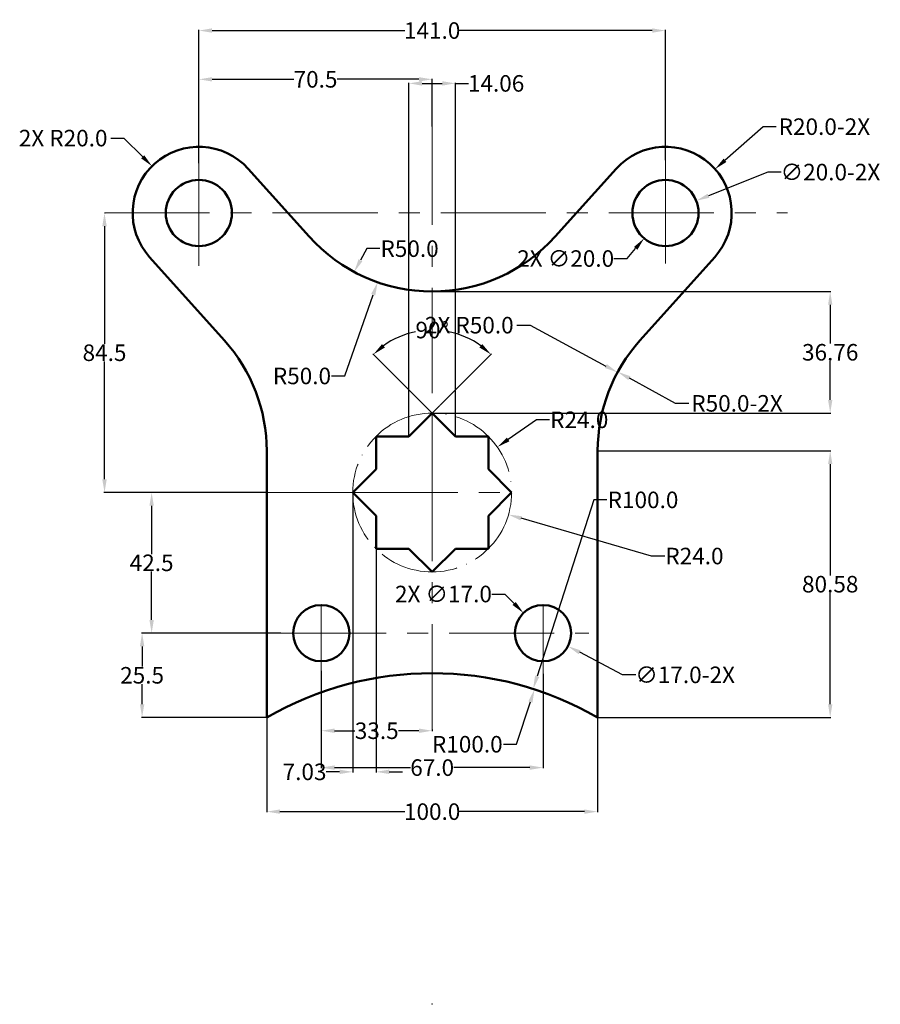
# Model space of a CAD drawing. Units: inches. Extents: x 181 to 441, y 19 to 317.
import ezdxf

# ---------------------------------------------------------------- set-up
doc = ezdxf.new("R2010")
doc.units = ezdxf.units.IN
doc.header["$MEASUREMENT"] = 0
doc.linetypes.add('ACAD_ISO04W100', pattern=[30, 24, -3, 0, -3])
doc.linetypes.add('CENTER', pattern=[50.8, 31.75, -6.35, 6.35, -6.35])
for name, color, linetype, lineweight in [('M-CNTR', 4, 'CENTER', 18), ('M-CONS', 4, 'ACAD_ISO04W100', 13), ('M-DIMS', 2, 'Continuous', 25), ('M-OUTL', 7, 'Continuous', 50)]:
    doc.layers.add(name, color=color, linetype=linetype, lineweight=lineweight)
doc.styles.get("Standard").update_dxf_attribs({"font": 'arial.ttf'})
doc.dimstyles.get("Standard").update_dxf_attribs({"dimtxt": 5, "dimasz": 4, "dimexe": 0.18, "dimexo": 0.0625, "dimgap": 0.09, "dimtad": 0, "dimtih": 1, "dimtoh": 1, "dimdec": 1, "dimzin": 0, "dimdsep": 46, "dimtxsty": 'Standard', "dimcen": 0.09, "dimadec": 0, "dimazin": 0, "dimtfac": 1, "dimtdec": 1, "dimtofl": 0, "dimtmove": 0, "dimatfit": 3, "dimfxl": 1, "dimtolj": 1, "dimtzin": 0, "dimarcsym": 0})

# ---------------------------------------------------------------- blocks, each defined once
blk = doc.blocks.new('*D1')
at = {"layer": 'Defpoints', "color": 0, "transparency": 16777216}
for p in [(336.36, 114.2), (305.44, 19.1)]:
    blk.add_point(p, dxfattribs=at)
at = {"layer": 'M-DIMS', "color": 0, "lineweight": -2, "transparency": 16777216}
for p, q in [((330.97, 97.61), (335.12, 110.39)), ((326.97, 97.61), (330.97, 97.61))]:
    blk.add_line(p, q, dxfattribs=at)
at = {"layer": 'M-DIMS', "color": 0, "transparency": 16777216}
blk.add_solid([(334.49, 110.6), (335.75, 110.19), (336.36, 114.2)], dxfattribs=at)
at = {"layer": 'M-DIMS', "color": 0, "transparency": 16777216, "insert": (316.06, 97.61), "char_height": 5, "attachment_point": 5}
blk.add_mtext('\\A1;R100.0', dxfattribs=at)
blk = doc.blocks.new('*D2')
at = {"layer": 'Defpoints', "color": 0, "transparency": 16777216}
for p in [(271.94, 119.92), (271.94, 101.7), (305.44, 102.17)]:
    blk.add_point(p, dxfattribs=at)
at = {"layer": 'M-DIMS', "color": 0, "lineweight": -2, "transparency": 16777216}
for p, q in [((271.94, 119.85), (271.94, 101.52)), ((275.94, 101.7), (282.09, 101.7)), ((301.44, 101.7), (295.29, 101.7)), ((305.44, 102.11), (305.44, 101.52))]:
    blk.add_line(p, q, dxfattribs=at)
at = {"layer": 'M-DIMS', "color": 0, "transparency": 16777216}
for points in [[(275.94, 102.36), (275.94, 101.03), (271.94, 101.7)], [(301.44, 102.36), (301.44, 101.03), (305.44, 101.7)]]:
    blk.add_solid(points, dxfattribs=at)
at = {"layer": 'M-DIMS', "color": 0, "transparency": 16777216, "insert": (288.69, 101.7), "char_height": 5, "attachment_point": 5}
blk.add_mtext('\\A1;33.5', dxfattribs=at)
blk = doc.blocks.new('*D3')
at = {"layer": 'Defpoints', "color": 0, "transparency": 16777216}
for p in [(271.94, 119.92), (338.94, 118.97), (338.94, 90.55)]:
    blk.add_point(p, dxfattribs=at)
at = {"layer": 'M-DIMS', "color": 0, "lineweight": -2, "transparency": 16777216}
for p, q in [((271.94, 119.85), (271.94, 90.37)), ((338.94, 118.91), (338.94, 90.37)), ((275.94, 90.55), (298.85, 90.55)), ((334.94, 90.55), (312.03, 90.55))]:
    blk.add_line(p, q, dxfattribs=at)
at = {"layer": 'M-DIMS', "color": 0, "transparency": 16777216}
for points in [[(275.94, 91.22), (275.94, 89.89), (271.94, 90.55)], [(334.94, 91.22), (334.94, 89.89), (338.94, 90.55)]]:
    blk.add_solid(points, dxfattribs=at)
at = {"layer": 'M-DIMS', "color": 0, "transparency": 16777216, "insert": (305.44, 90.55), "char_height": 5, "attachment_point": 5}
blk.add_mtext('\\A1;67.0', dxfattribs=at)
blk = doc.blocks.new('*D4')
at = {"layer": 'Defpoints', "color": 0, "transparency": 16777216}
for p in [(255.44, 105.7), (355.44, 105.7), (355.44, 77.24)]:
    blk.add_point(p, dxfattribs=at)
at = {"layer": 'M-DIMS', "color": 0, "lineweight": -2, "transparency": 16777216}
for p, q in [((255.44, 105.64), (255.44, 77.06)), ((355.44, 105.64), (355.44, 77.06)), ((259.44, 77.24), (297.16, 77.24)), ((351.44, 77.24), (313.73, 77.24))]:
    blk.add_line(p, q, dxfattribs=at)
at = {"layer": 'M-DIMS', "color": 0, "transparency": 16777216}
for points in [[(259.44, 77.91), (259.44, 76.58), (255.44, 77.24)], [(351.44, 77.91), (351.44, 76.58), (355.44, 77.24)]]:
    blk.add_solid(points, dxfattribs=at)
at = {"layer": 'M-DIMS', "color": 0, "transparency": 16777216, "insert": (305.44, 77.24), "char_height": 5, "attachment_point": 5}
blk.add_mtext('\\A1;100.0', dxfattribs=at)
blk = doc.blocks.new('*D5')
at = {"layer": 'Defpoints', "color": 0, "transparency": 16777216}
for p in [(331.41, 135.14), (346.47, 127.25)]:
    blk.add_point(p, dxfattribs=at)
at = {"layer": 'M-DIMS', "color": 0, "lineweight": -2, "transparency": 16777216}
for p, q in [((338.85, 131.2), (339.03, 131.2)), ((338.94, 131.11), (338.94, 131.29)), ((363, 118.59), (350.02, 125.4)), ((367, 118.59), (363, 118.59))]:
    blk.add_line(p, q, dxfattribs=at)
at = {"layer": 'M-DIMS', "color": 0, "transparency": 16777216}
blk.add_solid([(350.32, 125.99), (349.71, 124.81), (346.47, 127.25)], dxfattribs=at)
at = {"layer": 'M-DIMS', "color": 0, "transparency": 16777216, "insert": (381.88, 118.59), "char_height": 5, "attachment_point": 5}
blk.add_mtext('\\A1;∅17.0-2X', dxfattribs=at)
blk = doc.blocks.new('*D6')
at = {"layer": 'Defpoints', "color": 0, "transparency": 16777216}
for p in [(217.79, 131.2), (259.75, 131.2), (255.44, 105.7)]:
    blk.add_point(p, dxfattribs=at)
at = {"layer": 'M-DIMS', "color": 0, "lineweight": -2, "transparency": 16777216}
for p, q in [((259.69, 131.2), (217.61, 131.2)), ((217.79, 127.2), (217.79, 121.09)), ((217.79, 109.7), (217.79, 115.81)), ((255.38, 105.7), (217.61, 105.7))]:
    blk.add_line(p, q, dxfattribs=at)
at = {"layer": 'M-DIMS', "color": 0, "transparency": 16777216}
for points in [[(217.13, 127.2), (218.46, 127.2), (217.79, 131.2)], [(217.13, 109.7), (218.46, 109.7), (217.79, 105.7)]]:
    blk.add_solid(points, dxfattribs=at)
at = {"layer": 'M-DIMS', "color": 0, "transparency": 16777216, "insert": (217.79, 118.45), "char_height": 5, "attachment_point": 5}
blk.add_mtext('\\A1;25.5', dxfattribs=at)
blk = doc.blocks.new('*D7')
at = {"layer": 'Defpoints', "color": 0, "transparency": 16777216}
for p in [(220.67, 173.7), (255.44, 173.7), (259.75, 131.2)]:
    blk.add_point(p, dxfattribs=at)
at = {"layer": 'M-DIMS', "color": 0, "lineweight": -2, "transparency": 16777216}
for p, q in [((255.38, 173.7), (220.49, 173.7)), ((220.67, 169.7), (220.67, 155.09)), ((220.67, 135.2), (220.67, 149.81)), ((259.69, 131.2), (220.49, 131.2))]:
    blk.add_line(p, q, dxfattribs=at)
at = {"layer": 'M-DIMS', "color": 0, "transparency": 16777216}
for points in [[(220, 169.7), (221.34, 169.7), (220.67, 173.7)], [(220, 135.2), (221.34, 135.2), (220.67, 131.2)]]:
    blk.add_solid(points, dxfattribs=at)
at = {"layer": 'M-DIMS', "color": 0, "transparency": 16777216, "insert": (220.67, 152.45), "char_height": 5, "attachment_point": 5}
blk.add_mtext('\\A1;42.5', dxfattribs=at)
blk = doc.blocks.new('*D8')
at = {"layer": 'Defpoints', "color": 0, "transparency": 16777216}
for p in [(206.43, 258.2), (206.43, 258.2), (255.44, 173.7)]:
    blk.add_point(p, dxfattribs=at)
at = {"layer": 'M-DIMS', "color": 0, "lineweight": -2, "transparency": 16777216}
for p, q in [((206.49, 258.2), (206.61, 258.2)), ((206.43, 254.2), (206.43, 218.59)), ((206.43, 177.7), (206.43, 213.31)), ((255.38, 173.7), (206.25, 173.7))]:
    blk.add_line(p, q, dxfattribs=at)
at = {"layer": 'M-DIMS', "color": 0, "transparency": 16777216}
for points in [[(205.76, 254.2), (207.1, 254.2), (206.43, 258.2)], [(205.76, 177.7), (207.1, 177.7), (206.43, 173.7)]]:
    blk.add_solid(points, dxfattribs=at)
at = {"layer": 'M-DIMS', "color": 0, "transparency": 16777216, "insert": (206.43, 215.95), "char_height": 5, "attachment_point": 5}
blk.add_mtext('\\A1;84.5', dxfattribs=at)
blk = doc.blocks.new('*D9')
at = {"layer": 'Defpoints', "color": 0, "transparency": 16777216}
for p in [(305.44, 173.7), (328.5, 167.02)]:
    blk.add_point(p, dxfattribs=at)
at = {"layer": 'M-DIMS', "color": 0, "lineweight": -2, "transparency": 16777216}
for p, q in [((305.35, 173.7), (305.53, 173.7)), ((305.44, 173.61), (305.44, 173.79)), ((371.73, 154.5), (332.34, 165.91)), ((375.73, 154.5), (371.73, 154.5))]:
    blk.add_line(p, q, dxfattribs=at)
at = {"layer": 'M-DIMS', "color": 0, "transparency": 16777216}
blk.add_solid([(332.52, 166.55), (332.15, 165.27), (328.5, 167.02)], dxfattribs=at)
at = {"layer": 'M-DIMS', "color": 0, "transparency": 16777216, "insert": (384.7, 154.5), "char_height": 5, "attachment_point": 5}
blk.add_mtext('\\A1;R24.0', dxfattribs=at)
blk = doc.blocks.new('*D10')
at = {"layer": 'Defpoints', "color": 0, "transparency": 16777216}
for p in [(361.52, 210.17), (405.44, 186.28)]:
    blk.add_point(p, dxfattribs=at)
at = {"layer": 'M-DIMS', "color": 0, "lineweight": -2, "transparency": 16777216}
for p, q in [((379.02, 200.65), (365.03, 208.26)), ((383.02, 200.65), (379.02, 200.65))]:
    blk.add_line(p, q, dxfattribs=at)
at = {"layer": 'M-DIMS', "color": 0, "transparency": 16777216}
blk.add_solid([(365.35, 208.85), (364.72, 207.67), (361.52, 210.17)], dxfattribs=at)
at = {"layer": 'M-DIMS', "color": 0, "transparency": 16777216, "insert": (397.57, 200.65), "char_height": 5, "attachment_point": 5}
blk.add_mtext('\\A1;R50.0-2X', dxfattribs=at)
blk = doc.blocks.new('*D11')
at = {"layer": 'Defpoints', "color": 0, "transparency": 16777216}
for p in [(390.92, 271.45), (375.94, 258.2)]:
    blk.add_point(p, dxfattribs=at)
at = {"layer": 'M-DIMS', "color": 0, "lineweight": -2, "transparency": 16777216}
for p, q in [((405.42, 284.28), (393.92, 274.1)), ((409.42, 284.28), (405.42, 284.28)), ((375.85, 258.2), (376.03, 258.2)), ((375.94, 258.11), (375.94, 258.29))]:
    blk.add_line(p, q, dxfattribs=at)
at = {"layer": 'M-DIMS', "color": 0, "transparency": 16777216}
blk.add_solid([(393.48, 274.6), (394.36, 273.6), (390.92, 271.45)], dxfattribs=at)
at = {"layer": 'M-DIMS', "color": 0, "transparency": 16777216, "insert": (423.97, 284.28), "char_height": 5, "attachment_point": 5}
blk.add_mtext('\\A1;R20.0-2X', dxfattribs=at)
blk = doc.blocks.new('*D12')
at = {"layer": 'Defpoints', "color": 0, "transparency": 16777216}
for p in [(385.23, 261.9), (366.65, 254.49)]:
    blk.add_point(p, dxfattribs=at)
at = {"layer": 'M-DIMS', "color": 0, "lineweight": -2, "transparency": 16777216}
for p, q in [((406.91, 270.55), (388.95, 263.38)), ((410.91, 270.55), (406.91, 270.55)), ((375.85, 258.2), (376.03, 258.2)), ((375.94, 258.11), (375.94, 258.29))]:
    blk.add_line(p, q, dxfattribs=at)
at = {"layer": 'M-DIMS', "color": 0, "transparency": 16777216}
blk.add_solid([(388.7, 264), (389.19, 262.77), (385.23, 261.9)], dxfattribs=at)
at = {"layer": 'M-DIMS', "color": 0, "transparency": 16777216, "insert": (425.79, 270.55), "char_height": 5, "attachment_point": 5}
blk.add_mtext('\\A1;∅20.0-2X', dxfattribs=at)
blk = doc.blocks.new('*D13')
at = {"layer": 'Defpoints', "color": 0, "transparency": 16777216}
for p in [(305.44, 298.59), (305.44, 284.46), (234.94, 273.14)]:
    blk.add_point(p, dxfattribs=at)
at = {"layer": 'M-DIMS', "color": 0, "lineweight": -2, "transparency": 16777216}
for p, q in [((234.94, 273.2), (234.94, 298.77)), ((238.94, 298.59), (263.61, 298.59)), ((301.44, 298.59), (276.78, 298.59)), ((305.44, 284.52), (305.44, 298.77))]:
    blk.add_line(p, q, dxfattribs=at)
at = {"layer": 'M-DIMS', "color": 0, "transparency": 16777216}
for points in [[(238.94, 299.25), (238.94, 297.92), (234.94, 298.59)], [(301.44, 299.25), (301.44, 297.92), (305.44, 298.59)]]:
    blk.add_solid(points, dxfattribs=at)
at = {"layer": 'M-DIMS', "color": 0, "transparency": 16777216, "insert": (270.19, 298.59), "char_height": 5, "attachment_point": 5}
blk.add_mtext('\\A1;70.5', dxfattribs=at)
blk = doc.blocks.new('*D14')
at = {"layer": 'Defpoints', "color": 0, "transparency": 16777216}
for p in [(375.94, 313.33), (375.94, 274.13), (234.94, 273.14)]:
    blk.add_point(p, dxfattribs=at)
at = {"layer": 'M-DIMS', "color": 0, "lineweight": -2, "transparency": 16777216}
for p, q in [((234.94, 273.2), (234.94, 313.51)), ((238.94, 313.33), (297.16, 313.33)), ((371.94, 313.33), (313.73, 313.33)), ((375.94, 274.19), (375.94, 313.51))]:
    blk.add_line(p, q, dxfattribs=at)
at = {"layer": 'M-DIMS', "color": 0, "transparency": 16777216}
for points in [[(238.94, 314), (238.94, 312.67), (234.94, 313.33)], [(371.94, 314), (371.94, 312.67), (375.94, 313.33)]]:
    blk.add_solid(points, dxfattribs=at)
at = {"layer": 'M-DIMS', "color": 0, "transparency": 16777216, "insert": (305.44, 313.33), "char_height": 5, "attachment_point": 5}
blk.add_mtext('\\A1;141.0', dxfattribs=at)
blk = doc.blocks.new('*D15')
at = {"layer": 'Defpoints', "color": 0, "transparency": 16777216}
for p in [(305.44, 284.46), (281.88, 240.36)]:
    blk.add_point(p, dxfattribs=at)
at = {"layer": 'M-DIMS', "color": 0, "lineweight": -2, "transparency": 16777216}
for p, q in [((285.65, 247.41), (283.76, 243.89)), ((289.65, 247.41), (285.65, 247.41))]:
    blk.add_line(p, q, dxfattribs=at)
at = {"layer": 'M-DIMS', "color": 0, "transparency": 16777216}
blk.add_solid([(283.18, 244.2), (284.35, 243.57), (281.88, 240.36)], dxfattribs=at)
at = {"layer": 'M-DIMS', "color": 0, "transparency": 16777216, "insert": (298.62, 247.41), "char_height": 5, "attachment_point": 5}
blk.add_mtext('\\A1;R50.0', dxfattribs=at)
blk = doc.blocks.new('*D16')
at = {"layer": 'Defpoints', "color": 0, "transparency": 16777216}
for p in [(311.94, 221.95), (302.44, 200.7), (307.78, 200.03), (305.44, 197.7), (305.44, 197.7)]:
    blk.add_point(p, dxfattribs=at)
at = {"layer": 'M-DIMS', "color": 0, "lineweight": -2, "transparency": 16777216}
for p, q in [((302.4, 200.74), (287.56, 215.58)), ((307.82, 200.08), (323.33, 215.58))]:
    blk.add_line(p, q, dxfattribs=at)
for start, end in [(101.4724, 125.8636), (54.1364, 78.5276)]:
    blk.add_arc((305.44, 197.7), 25.11, start, end, dxfattribs=at)
at = {"layer": 'M-DIMS', "color": 0, "transparency": 16777216}
for points in [[(291.16, 217.54), (290.3, 218.56), (287.69, 215.45)], [(320.59, 218.56), (319.72, 217.54), (323.2, 215.45)]]:
    blk.add_solid(points, dxfattribs=at)
at = {"layer": 'M-DIMS', "color": 0, "transparency": 16777216, "insert": (305.44, 222.81), "char_height": 5, "attachment_point": 5}
blk.add_mtext('\\A1;90°', dxfattribs=at)
blk = doc.blocks.new('MOUNT-HOLE-D17')
blk.add_circle((0, 0), 8.5)
blk = doc.blocks.new('ANCHOR-HOLE-D20')
blk.add_circle((0, 0), 10)
blk = doc.blocks.new('*D19')
at = {"layer": 'Defpoints', "color": 0, "transparency": 16777216}
for p in [(355.44, 186.28), (425.72, 186.28), (355.44, 105.7)]:
    blk.add_point(p, dxfattribs=at)
at = {"layer": 'M-DIMS', "color": 0, "lineweight": -2, "transparency": 16777216}
for p, q in [((355.51, 186.28), (425.9, 186.28)), ((425.72, 182.28), (425.72, 148.63)), ((425.72, 109.7), (425.72, 143.35)), ((355.51, 105.7), (425.9, 105.7))]:
    blk.add_line(p, q, dxfattribs=at)
at = {"layer": 'M-DIMS', "color": 0, "transparency": 16777216}
for points in [[(425.06, 182.28), (426.39, 182.28), (425.72, 186.28)], [(425.06, 109.7), (426.39, 109.7), (425.72, 105.7)]]:
    blk.add_solid(points, dxfattribs=at)
at = {"layer": 'M-DIMS', "color": 0, "transparency": 16777216, "insert": (425.72, 145.99), "char_height": 5, "attachment_point": 5}
blk.add_mtext('\\A1;80.58', dxfattribs=at)
blk = doc.blocks.new('*D20')
at = {"layer": 'Defpoints', "color": 0, "transparency": 16777216}
for p in [(305.44, 234.46), (305.44, 197.7), (425.72, 197.7)]:
    blk.add_point(p, dxfattribs=at)
at = {"layer": 'M-DIMS', "color": 0, "lineweight": -2, "transparency": 16777216}
for p, q in [((305.51, 234.46), (425.9, 234.46)), ((425.72, 230.46), (425.72, 218.72)), ((425.72, 201.7), (425.72, 213.43)), ((305.51, 197.7), (425.9, 197.7))]:
    blk.add_line(p, q, dxfattribs=at)
at = {"layer": 'M-DIMS', "color": 0, "transparency": 16777216}
for points in [[(425.06, 230.46), (426.39, 230.46), (425.72, 234.46)], [(425.06, 201.7), (426.39, 201.7), (425.72, 197.7)]]:
    blk.add_solid(points, dxfattribs=at)
at = {"layer": 'M-DIMS', "color": 0, "transparency": 16777216, "insert": (425.72, 216.08), "char_height": 5, "attachment_point": 5}
blk.add_mtext('\\A1;36.76', dxfattribs=at)
blk = doc.blocks.new('*D21')
at = {"layer": 'Defpoints', "color": 0, "transparency": 16777216}
for p in [(312.47, 297.36), (298.41, 190.67), (312.47, 190.67)]:
    blk.add_point(p, dxfattribs=at)
at = {"layer": 'M-DIMS', "color": 0, "lineweight": -2, "transparency": 16777216}
for p, q in [((298.41, 190.73), (298.41, 297.54)), ((302.41, 297.36), (308.47, 297.36)), ((312.47, 190.73), (312.47, 297.54)), ((312.47, 297.36), (316.47, 297.36))]:
    blk.add_line(p, q, dxfattribs=at)
at = {"layer": 'M-DIMS', "color": 0, "transparency": 16777216}
for points in [[(302.41, 298.02), (302.41, 296.69), (298.41, 297.36)], [(308.47, 298.02), (308.47, 296.69), (312.47, 297.36)]]:
    blk.add_solid(points, dxfattribs=at)
at = {"layer": 'M-DIMS', "color": 0, "transparency": 16777216, "insert": (324.76, 297.36), "char_height": 5, "attachment_point": 5}
blk.add_mtext('\\A1;14.06', dxfattribs=at)
blk = doc.blocks.new('*D22')
at = {"layer": 'Defpoints', "color": 0, "transparency": 16777216}
for p in [(281.44, 173.7), (288.47, 166.67), (281.44, 89.27)]:
    blk.add_point(p, dxfattribs=at)
at = {"layer": 'M-DIMS', "color": 0, "lineweight": -2, "transparency": 16777216}
for p, q in [((281.44, 173.64), (281.44, 89.09)), ((288.47, 166.61), (288.47, 89.09)), ((277.44, 89.27), (273.44, 89.27)), ((292.47, 89.27), (296.47, 89.27))]:
    blk.add_line(p, q, dxfattribs=at)
at = {"layer": 'M-DIMS', "color": 0, "transparency": 16777216}
for points in [[(277.44, 89.94), (277.44, 88.6), (281.44, 89.27)], [(292.47, 89.94), (292.47, 88.6), (288.47, 89.27)]]:
    blk.add_solid(points, dxfattribs=at)
at = {"layer": 'M-DIMS', "color": 0, "transparency": 16777216, "insert": (266.88, 89.27), "char_height": 5, "attachment_point": 5}
blk.add_mtext('\\A1;7.03', dxfattribs=at)
blk = doc.blocks.new('*D23')
at = {"layer": 'Defpoints', "color": 0, "transparency": 16777216}
for p in [(382.38, 265.85), (369.51, 250.55)]:
    blk.add_point(p, dxfattribs=at)
at = {"layer": 'M-DIMS', "color": 0, "lineweight": -2, "transparency": 16777216}
for p, q in [((375.85, 258.2), (376.03, 258.2)), ((375.94, 258.11), (375.94, 258.29)), ((364.35, 244.42), (366.93, 247.49)), ((360.35, 244.42), (364.35, 244.42))]:
    blk.add_line(p, q, dxfattribs=at)
at = {"layer": 'M-DIMS', "color": 0, "transparency": 16777216}
blk.add_solid([(366.42, 247.91), (367.44, 247.06), (369.51, 250.55)], dxfattribs=at)
at = {"layer": 'M-DIMS', "color": 0, "transparency": 16777216, "insert": (345.78, 244.42), "char_height": 5, "attachment_point": 5}
blk.add_mtext('\\A1;2X ∅20.0', dxfattribs=at)
blk = doc.blocks.new('*D24')
at = {"layer": 'Defpoints', "color": 0, "transparency": 16777216}
for p in [(333.01, 137.29), (344.87, 125.11)]:
    blk.add_point(p, dxfattribs=at)
at = {"layer": 'M-DIMS', "color": 0, "lineweight": -2, "transparency": 16777216}
for p, q in [((323.43, 143.02), (327.43, 143.02)), ((327.43, 143.02), (330.22, 140.15)), ((338.85, 131.2), (339.03, 131.2)), ((338.94, 131.11), (338.94, 131.29))]:
    blk.add_line(p, q, dxfattribs=at)
at = {"layer": 'M-DIMS', "color": 0, "transparency": 16777216}
blk.add_solid([(330.7, 140.62), (329.74, 139.69), (333.01, 137.29)], dxfattribs=at)
at = {"layer": 'M-DIMS', "color": 0, "transparency": 16777216, "insert": (308.85, 143.02), "char_height": 5, "attachment_point": 5}
blk.add_mtext('\\A1;2X ∅17.0', dxfattribs=at)
blk = doc.blocks.new('*D25')
at = {"layer": 'Defpoints', "color": 0, "transparency": 16777216}
for p in [(220.8, 272.34), (234.94, 258.2)]:
    blk.add_point(p, dxfattribs=at)
at = {"layer": 'M-DIMS', "color": 0, "lineweight": -2, "transparency": 16777216}
for p, q in [((208.31, 280.82), (212.31, 280.82)), ((212.31, 280.82), (217.97, 275.17)), ((234.85, 258.2), (235.03, 258.2)), ((234.94, 258.11), (234.94, 258.29))]:
    blk.add_line(p, q, dxfattribs=at)
at = {"layer": 'M-DIMS', "color": 0, "transparency": 16777216}
blk.add_solid([(218.44, 275.64), (217.5, 274.7), (220.8, 272.34)], dxfattribs=at)
at = {"layer": 'M-DIMS', "color": 0, "transparency": 16777216, "insert": (193.93, 280.82), "char_height": 5, "attachment_point": 5}
blk.add_mtext('\\A1;2X R20.0', dxfattribs=at)
blk = doc.blocks.new('*D26')
at = {"layer": 'Defpoints', "color": 0, "transparency": 16777216}
for p in [(325.12, 187.44), (305.44, 173.7)]:
    blk.add_point(p, dxfattribs=at)
at = {"layer": 'M-DIMS', "color": 0, "lineweight": -2, "transparency": 16777216}
for p, q in [((336.93, 195.68), (328.4, 189.73)), ((340.93, 195.68), (336.93, 195.68)), ((305.35, 173.7), (305.53, 173.7)), ((305.44, 173.61), (305.44, 173.79))]:
    blk.add_line(p, q, dxfattribs=at)
at = {"layer": 'M-DIMS', "color": 0, "transparency": 16777216}
blk.add_solid([(328.02, 190.28), (328.78, 189.18), (325.12, 187.44)], dxfattribs=at)
at = {"layer": 'M-DIMS', "color": 0, "transparency": 16777216, "insert": (349.89, 195.68), "char_height": 5, "attachment_point": 5}
blk.add_mtext('\\A1;R24.0', dxfattribs=at)
blk = doc.blocks.new('*D27')
at = {"layer": 'Defpoints', "color": 0, "transparency": 16777216}
for p in [(305.44, 284.46), (288.95, 237.26)]:
    blk.add_point(p, dxfattribs=at)
at = {"layer": 'M-DIMS', "color": 0, "lineweight": -2, "transparency": 16777216}
for p, q in [((305.35, 284.46), (305.53, 284.46)), ((305.44, 284.37), (305.44, 284.55)), ((279.05, 208.93), (287.63, 233.48)), ((275.05, 208.93), (279.05, 208.93))]:
    blk.add_line(p, q, dxfattribs=at)
at = {"layer": 'M-DIMS', "color": 0, "transparency": 16777216}
blk.add_solid([(287, 233.7), (288.26, 233.26), (288.95, 237.26)], dxfattribs=at)
at = {"layer": 'M-DIMS', "color": 0, "transparency": 16777216, "insert": (266.09, 208.93), "char_height": 5, "attachment_point": 5}
blk.add_mtext('\\A1;R50.0', dxfattribs=at)
blk = doc.blocks.new('*D28')
at = {"layer": 'Defpoints', "color": 0, "transparency": 16777216}
for p in [(361.44, 210.03), (405.44, 186.28)]:
    blk.add_point(p, dxfattribs=at)
at = {"layer": 'M-DIMS', "color": 0, "lineweight": -2, "transparency": 16777216}
for p, q in [((331.05, 224.28), (335.05, 224.28)), ((335.05, 224.28), (357.92, 211.93)), ((405.35, 186.28), (405.53, 186.28)), ((405.44, 186.19), (405.44, 186.37))]:
    blk.add_line(p, q, dxfattribs=at)
at = {"layer": 'M-DIMS', "color": 0, "transparency": 16777216}
blk.add_solid([(358.24, 212.52), (357.61, 211.34), (361.44, 210.03)], dxfattribs=at)
at = {"layer": 'M-DIMS', "color": 0, "transparency": 16777216, "insert": (316.66, 224.28), "char_height": 5, "attachment_point": 5}
blk.add_mtext('\\A1;2X R50.0', dxfattribs=at)
blk = doc.blocks.new('*D29')
at = {"layer": 'Defpoints', "color": 0, "transparency": 16777216}
for p in [(335.95, 114.33), (305.44, 19.1)]:
    blk.add_point(p, dxfattribs=at)
at = {"layer": 'M-DIMS', "color": 0, "lineweight": -2, "transparency": 16777216}
for p, q in [((354.25, 171.47), (337.17, 118.14)), ((358.25, 171.47), (354.25, 171.47)), ((305.35, 19.1), (305.53, 19.1)), ((305.44, 19.01), (305.44, 19.19))]:
    blk.add_line(p, q, dxfattribs=at)
at = {"layer": 'M-DIMS', "color": 0, "transparency": 16777216}
blk.add_solid([(336.53, 118.34), (337.8, 117.93), (335.95, 114.33)], dxfattribs=at)
at = {"layer": 'M-DIMS', "color": 0, "transparency": 16777216, "insert": (369.16, 171.47), "char_height": 5, "attachment_point": 5}
blk.add_mtext('\\A1;R100.0', dxfattribs=at)

msp = doc.modelspace()

# ---------------------------------------------------------------- linework, layer by layer
at = {"layer": 'M-CNTR'}
for p, q in [((305.443, 102.171), (305.443, 284.457)), ((375.943, 242.935), (375.943, 274.125)), ((234.943, 242.192), (234.943, 273.135)), ((206.429, 258.198), (412.822, 258.198)), ((305.443, 197.698), (305.443, 149.698)), ((281.443, 173.698), (255.443, 173.698)), ((281.443, 173.698), (329.443, 173.698)), ((271.943, 119.916), (271.943, 139.698)), ((338.943, 118.975), (338.943, 139.698)), ((259.75, 131.198), (352.828, 131.198))]:
    msp.add_line(p, q, dxfattribs=at)
at = {"layer": 'M-CONS'}
for q in [(302.443, 200.698), (307.78, 200.034)]:
    msp.add_line((305.443, 197.698), q, dxfattribs=at)
msp.add_circle((305.443, 173.698), 24, dxfattribs=at)
at = {"layer": 'M-OUTL'}
for p, q in [((249.824, 271.56), (268.24, 251.051)), ((361.062, 271.56), (342.646, 251.051)), ((220.062, 244.836), (242.646, 219.685)), ((390.824, 244.836), (368.24, 219.685)), ((298.414, 190.669), (305.443, 197.698)), ((305.443, 197.698), (312.473, 190.669)), ((288.473, 190.669), (288.473, 180.727)), ((298.414, 190.669), (288.473, 190.669)), ((322.414, 190.669), (312.473, 190.669)), ((322.414, 190.669), (322.414, 180.727)), ((255.443, 173.698), (255.443, 186.279)), ((355.443, 173.698), (355.443, 186.279)), ((281.443, 173.698), (288.473, 180.727)), ((322.414, 180.727), (329.443, 173.698)), ((255.443, 131.198), (255.443, 173.698)), ((288.473, 166.669), (281.443, 173.698)), ((329.443, 173.698), (322.414, 166.669)), ((355.443, 173.698), (355.443, 131.198)), ((288.473, 166.669), (288.473, 156.727)), ((322.414, 166.669), (322.414, 156.727)), ((298.414, 156.727), (288.473, 156.727)), ((305.443, 149.698), (298.414, 156.727)), ((312.473, 156.727), (305.443, 149.698)), ((322.414, 156.727), (312.473, 156.727)), ((255.443, 105.698), (255.443, 131.198)), ((355.443, 131.198), (355.443, 105.698))]:
    msp.add_line(p, q, dxfattribs=at)
for centre, radius, start, end in [((234.943, 258.198), 20, 41.92194, 221.92194), ((375.943, 258.198), 20, 318.07806, 138.07806), ((305.443, 284.457), 50, 221.92194, 318.07806), ((205.443, 186.279), 50, 0, 41.92194), ((405.443, 186.279), 50, 138.07806, 180), ((305.443, 19.095), 100, 60, 120)]:
    msp.add_arc(centre, radius, start, end, dxfattribs=at)

# ---------------------------------------------------------------- block references
for name, p in [('ANCHOR-HOLE-D20', (234.943, 258.198)), ('ANCHOR-HOLE-D20', (375.943, 258.198)), ('MOUNT-HOLE-D17', (271.943, 131.198)), ('MOUNT-HOLE-D17', (338.943, 131.198))]:
    msp.add_blockref(name, p, dxfattribs=at)

# ---------------------------------------------------------------- dimensions: what is measured, and where the dimension line sits
at = {"layer": 'M-DIMS'}
for base, p1, p2, override, picture, middle in [((375.943, 313.334), (234.943, 273.135), (375.943, 274.125), {"dimclrd": 0, "dimclre": 0, "dimclrt": 0}, '*D14', (305.443, 313.334)), ((305.443, 298.587), (234.943, 273.135), (305.443, 284.457), {"dimclrd": 0, "dimclre": 0, "dimclrt": 0}, '*D13', (270.193, 298.587)), ((312.473, 297.357), (298.414, 190.669), (312.473, 190.669), {"dimdec": 2, "dimlfac": 1, "dimrnd": 0, "dimzin": 0, "dimdsep": 46, "dimlunit": 2}, '*D21', (324.762, 297.357)), ((281.443, 89.271), (288.473, 166.669), (281.443, 173.698), {"dimdec": 2, "dimlfac": 1, "dimrnd": 0, "dimzin": 0, "dimdsep": 46, "dimlunit": 2}, '*D22', (266.88, 89.271)), ((271.943, 101.696), (305.443, 102.171), (271.943, 119.916), {"dimclrd": 0, "dimclre": 0, "dimclrt": 0}, '*D2', (288.693, 101.696)), ((338.943, 90.552), (271.943, 119.916), (338.943, 118.975), {"dimclrd": 0, "dimclre": 0, "dimclrt": 0}, '*D3', (305.443, 90.552)), ((355.443, 77.243), (255.443, 105.698), (355.443, 105.698), {"dimclrd": 0, "dimclre": 0, "dimclrt": 0}, '*D4', (305.443, 77.243))]:
    dim = msp.add_linear_dim(base=base, p1=p1, p2=p2, dimstyle='Standard', override=override, dxfattribs=at)
    dim.commit()
    dim.dimension.update_dxf_attribs({"geometry": picture, "text_midpoint": middle})
for center, mpoint, text, override, picture, middle in [((234.943, 258.198), (220.8, 272.34), '2X <>', {"dimdec": 1, "dimlfac": 1, "dimrnd": 0, "dimzin": 0, "dimdsep": 46, "dimlunit": 2}, '*D25', (193.932, 280.825)), ((375.943, 258.198), (390.921, 271.452), '<>-2X', {"dimclrd": 0, "dimclre": 0, "dimclrt": 0}, '*D11', (423.966, 284.279)), ((405.443, 186.279), (361.444, 210.03), '2X <>', {"dimdec": 1, "dimlfac": 1, "dimrnd": 0, "dimzin": 0, "dimdsep": 46, "dimlunit": 2}, '*D28', (316.663, 224.281)), ((405.443, 186.279), (361.521, 210.171), '<>-2X', {"dimclrd": 0, "dimclre": 0, "dimclrt": 0}, '*D10', (397.567, 200.653))]:
    dim = msp.add_radius_dim(center=center, mpoint=mpoint, text=text, dimstyle='Standard', override=override, dxfattribs=at)
    dim.commit()
    dim.dimension.update_dxf_attribs({"geometry": picture, "text_midpoint": middle, "dimtype": 164})
for center, mpoint, override, picture, middle in [((305.443, 284.457), (288.95, 237.256), {"dimdec": 1, "dimlfac": 1, "dimrnd": 0, "dimzin": 0, "dimdsep": 46, "dimlunit": 2}, '*D27', (266.086, 208.935)), ((305.443, 284.457), (281.878, 240.358), {"dimclrd": 0, "dimclre": 0, "dimclrt": 0}, '*D15', (298.616, 247.414)), ((305.443, 173.698), (325.12, 187.44), {"dimdec": 1, "dimlfac": 1, "dimrnd": 0, "dimzin": 0, "dimdsep": 46, "dimlunit": 2}, '*D26', (349.893, 195.685)), ((305.443, 19.095), (335.949, 114.329), {"dimdec": 1, "dimlfac": 1, "dimrnd": 0, "dimzin": 0, "dimdsep": 46, "dimlunit": 2}, '*D29', (369.163, 171.469)), ((305.443, 173.698), (328.496, 167.022), {"dimclrd": 0, "dimclre": 0, "dimclrt": 0}, '*D9', (384.702, 154.499)), ((305.443, 19.095), (336.358, 114.197), {"dimclrd": 0, "dimclre": 0, "dimclrt": 0}, '*D1', (316.056, 97.611))]:
    dim = msp.add_radius_dim(center=center, mpoint=mpoint, dimstyle='Standard', override=override, dxfattribs=at)
    dim.commit()
    dim.dimension.update_dxf_attribs({"geometry": picture, "text_midpoint": middle, "dimtype": 164})
for p1, p2, text, override, picture, middle in [((366.655, 254.493), (385.231, 261.903), '<>-2X', {"dimclrd": 0, "dimclre": 0, "dimclrt": 0}, '*D12', (425.789, 270.551)), ((382.381, 265.85), (369.505, 250.546), '2X <>', {"dimdec": 1, "dimlfac": 1, "dimrnd": 0, "dimzin": 0, "dimdsep": 46, "dimlunit": 2}, '*D23', (345.778, 244.425)), ((344.874, 125.109), (333.012, 137.287), '2X <>', {"dimdec": 1, "dimlfac": 1, "dimrnd": 0, "dimzin": 0, "dimdsep": 46, "dimlunit": 2}, '*D24', (308.854, 143.018)), ((331.414, 135.143), (346.472, 127.253), '<>-2X', {"dimclrd": 0, "dimclre": 0, "dimclrt": 0}, '*D5', (381.879, 118.59))]:
    dim = msp.add_diameter_dim_2p(p1=p1, p2=p2, text=text, dimstyle='Standard', override=override, dxfattribs=at)
    dim.commit()
    dim.dimension.update_dxf_attribs({"geometry": picture, "text_midpoint": middle, "dimtype": 163})
for base, p1, p2, override, picture, middle in [((206.429, 258.198), (255.443, 173.698), (206.429, 258.198), {"dimclrd": 0, "dimclre": 0, "dimclrt": 0}, '*D8', (206.429, 215.948)), ((425.722, 197.698), (305.443, 234.457), (305.443, 197.698), {"dimdec": 2, "dimlfac": 1, "dimrnd": 0, "dimzin": 0, "dimdsep": 46, "dimlunit": 2}, '*D20', (425.722, 216.078)), ((425.722, 186.279), (355.443, 105.698), (355.443, 186.279), {"dimdec": 2, "dimlfac": 1, "dimrnd": 0, "dimzin": 0, "dimdsep": 46, "dimlunit": 2}, '*D19', (425.722, 145.989)), ((220.669, 173.698), (259.75, 131.198), (255.443, 173.698), {"dimclrd": 0, "dimclre": 0, "dimclrt": 0}, '*D7', (220.669, 152.448)), ((217.794, 131.198), (255.443, 105.698), (259.75, 131.198), {"dimclrd": 0, "dimclre": 0, "dimclrt": 0}, '*D6', (217.794, 118.448))]:
    dim = msp.add_linear_dim(base=base, p1=p1, p2=p2, angle=90, dimstyle='Standard', override=override, dxfattribs=at)
    dim.commit()
    dim.dimension.update_dxf_attribs({"geometry": picture, "text_midpoint": middle})
dim = msp.add_angular_dim_2l(base=(311.942, 221.954), line1=((305.443, 197.698), (307.78, 200.034)), line2=((305.443, 197.698), (302.443, 200.698)), dimstyle='Standard', override={"dimclrd": 0, "dimclre": 0, "dimclrt": 0}, dxfattribs=at)
dim.commit()
dim.dimension.update_dxf_attribs({"geometry": '*D16', "text_midpoint": (305.443, 222.809)})

doc.saveas('drawing.dxf')
